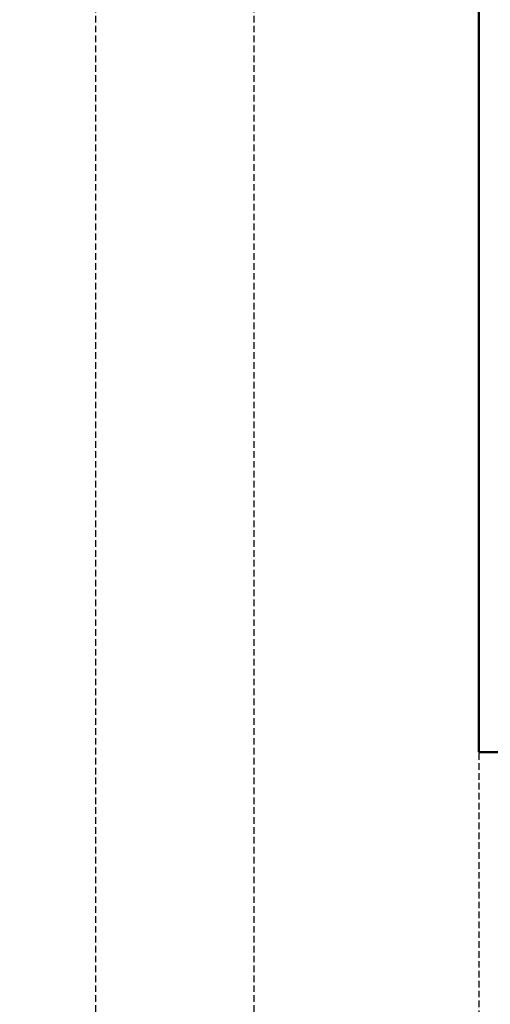
# Model space of a CAD drawing. Units: inches. Extents: x 513 to 1142, y 396 to 927.
# Tile 23 of 31: x 886 to 922, y 691 to 766. Entities that reach past the tile are written whole.
import ezdxf

# ---------------------------------------------------------------- set-up
doc = ezdxf.new("R2010")
doc.units = ezdxf.units.IN
doc.header["$MEASUREMENT"] = 0
doc.linetypes.add('DASHED', pattern=[0.75, 0.5, -0.25])
doc.layers.add('A-ANNO-DIMS', color=2, linetype='DASHED', lineweight=18)
doc.layers.add('A-WALL', color=7, linetype='Continuous', lineweight=50)
doc.styles.get("Standard").update_dxf_attribs({"font": 'arial.ttf'})
doc.dimstyles.get("Standard").update_dxf_attribs({"dimtxt": 4, "dimasz": 0.18, "dimexe": 0.18, "dimexo": 0.0625, "dimgap": 0.09, "dimtad": 0, "dimtih": 1, "dimtoh": 1, "dimdec": 0, "dimrnd": 6, "dimzin": 0, "dimdsep": 46, "dimlunit": 3, "dimtxsty": 'Standard', "dimcen": 0.09, "dimadec": 0, "dimazin": 0, "dimtfac": 1, "dimtdec": 0, "dimtofl": 0, "dimtmove": 0, "dimatfit": 3, "dimfxl": 1, "dimtolj": 1, "dimtzin": 0, "dimarcsym": 0})

# ---------------------------------------------------------------- blocks, each defined once
blk = doc.blocks.new('*D137')
at = {"layer": 'A-ANNO-DIMS', "color": 0, "lineweight": -2, "transparency": 16777216}
for p, q in [((839.995, 770.096), (839.995, 401.578)), ((920.995, 770.067), (920.995, 401.578)), ((840.175, 401.758), (875.078, 401.758)), ((920.815, 401.758), (885.913, 401.758))]:
    blk.add_line(p, q, dxfattribs=at)
at = {"layer": 'A-ANNO-DIMS', "color": 0, "transparency": 16777216}
for points in [[(840.175, 401.788), (840.175, 401.728), (839.995, 401.758)], [(920.815, 401.788), (920.815, 401.728), (920.995, 401.758)]]:
    blk.add_solid(points, dxfattribs=at)
at = {"layer": 'Defpoints', "color": 0, "transparency": 16777216}
for p in [(839.995, 770.158), (920.995, 770.13), (920.995, 401.758)]:
    blk.add_point(p, dxfattribs=at)
at = {"layer": 'A-ANNO-DIMS', "color": 0, "transparency": 16777216, "insert": (880.495, 401.758), "char_height": 4, "attachment_point": 5}
blk.add_mtext('\\A1;6\'-9"', dxfattribs=at)
blk = doc.blocks.new('*D149')
at = {"layer": 'A-ANNO-DIMS', "color": 0, "lineweight": -2, "transparency": 16777216}
for p, q in [((840.058, 770.158), (1131.575, 770.158)), ((1131.395, 769.978), (1131.395, 707.791)), ((1131.395, 641.338), (1131.395, 703.526)), ((840.058, 641.158), (1131.575, 641.158))]:
    blk.add_line(p, q, dxfattribs=at)
at = {"layer": 'A-ANNO-DIMS', "color": 0, "transparency": 16777216}
for points in [[(1131.365, 769.978), (1131.425, 769.978), (1131.395, 770.158)], [(1131.365, 641.338), (1131.425, 641.338), (1131.395, 641.158)]]:
    blk.add_solid(points, dxfattribs=at)
at = {"layer": 'Defpoints', "color": 0, "transparency": 16777216}
for p in [(839.995, 770.158), (1131.395, 770.158), (839.995, 641.158)]:
    blk.add_point(p, dxfattribs=at)
at = {"layer": 'A-ANNO-DIMS', "color": 0, "transparency": 16777216, "insert": (1131.395, 705.658), "char_height": 4, "attachment_point": 5}
blk.add_mtext('\\A1;10\'-9"', dxfattribs=at)
blk = doc.blocks.new('*D168')
at = {"layer": 'A-ANNO-DIMS', "color": 0, "lineweight": -2, "transparency": 16777216}
for p, q in [((891.995, 637.221), (891.995, 920.738)), ((892.175, 920.558), (892.777, 920.558)), ((903.815, 920.558), (903.214, 920.558)), ((903.995, 637.221), (903.995, 920.738))]:
    blk.add_line(p, q, dxfattribs=at)
at = {"layer": 'A-ANNO-DIMS', "color": 0, "transparency": 16777216}
for points in [[(892.175, 920.588), (892.175, 920.528), (891.995, 920.558)], [(903.815, 920.588), (903.815, 920.528), (903.995, 920.558)]]:
    blk.add_solid(points, dxfattribs=at)
at = {"layer": 'Defpoints', "color": 0, "transparency": 16777216}
for p in [(903.995, 920.558), (891.995, 637.158), (903.995, 637.158)]:
    blk.add_point(p, dxfattribs=at)
at = {"layer": 'A-ANNO-DIMS', "color": 0, "transparency": 16777216, "insert": (897.995, 920.558), "char_height": 4, "attachment_point": 5}
blk.add_mtext('\\A1;1\'-0"', dxfattribs=at)
blk = doc.blocks.new('*D176')
at = {"layer": 'A-ANNO-DIMS', "color": 0, "lineweight": -2, "transparency": 16777216}
for p, q in [((847.995, 637.221), (847.995, 920.738)), ((848.175, 920.558), (864.59, 920.558)), ((891.815, 920.558), (875.4, 920.558)), ((891.995, 637.221), (891.995, 920.738))]:
    blk.add_line(p, q, dxfattribs=at)
at = {"layer": 'A-ANNO-DIMS', "color": 0, "transparency": 16777216}
for points in [[(848.175, 920.588), (848.175, 920.528), (847.995, 920.558)], [(891.815, 920.588), (891.815, 920.528), (891.995, 920.558)]]:
    blk.add_solid(points, dxfattribs=at)
at = {"layer": 'Defpoints', "color": 0, "transparency": 16777216}
for p in [(891.995, 920.558), (847.995, 637.158), (891.995, 637.158)]:
    blk.add_point(p, dxfattribs=at)
at = {"layer": 'A-ANNO-DIMS', "color": 0, "transparency": 16777216, "insert": (869.995, 920.558), "char_height": 4, "attachment_point": 5}
blk.add_mtext('\\A1;3\'-8"', dxfattribs=at)

msp = doc.modelspace()

# ---------------------------------------------------------------- linework, layer by layer
at = {"layer": 'A-WALL'}
for p, q in [((920.995, 710.158), (920.995, 870.158)), ((924.995, 710.158), (920.995, 710.158))]:
    msp.add_line(p, q, dxfattribs=at)

# ---------------------------------------------------------------- dimensions: what is measured, and where the dimension line sits
at = {"layer": 'A-ANNO-DIMS'}
for base, p1, p2, picture, middle in [((891.995, 920.558), (847.995, 637.158), (891.995, 637.158), '*D176', (869.995, 920.558)), ((903.995, 920.558), (891.995, 637.158), (903.995, 637.158), '*D168', (897.995, 920.558)), ((920.995, 401.758), (839.995, 770.158), (920.995, 770.13), '*D137', (880.495, 401.758))]:
    dim = msp.add_linear_dim(base=base, p1=p1, p2=p2, dimstyle='Standard', override={"dimdec": 1, "dimlfac": 1, "dimrnd": 0, "dimzin": 1, "dimdsep": 46, "dimlunit": 4, "dimfrac": 2}, dxfattribs=at)
    dim.commit()
    dim.dimension.update_dxf_attribs({"geometry": picture, "text_midpoint": middle})
dim = msp.add_linear_dim(base=(1131.395, 770.158), p1=(839.995, 641.158), p2=(839.995, 770.158), angle=90, dimstyle='Standard', override={"dimdec": 1, "dimlfac": 1, "dimrnd": 0, "dimzin": 1, "dimdsep": 46, "dimlunit": 4, "dimfrac": 2}, dxfattribs=at)
dim.commit()
dim.dimension.update_dxf_attribs({"geometry": '*D149', "text_midpoint": (1131.395, 705.658)})

doc.saveas('drawing.dxf')
